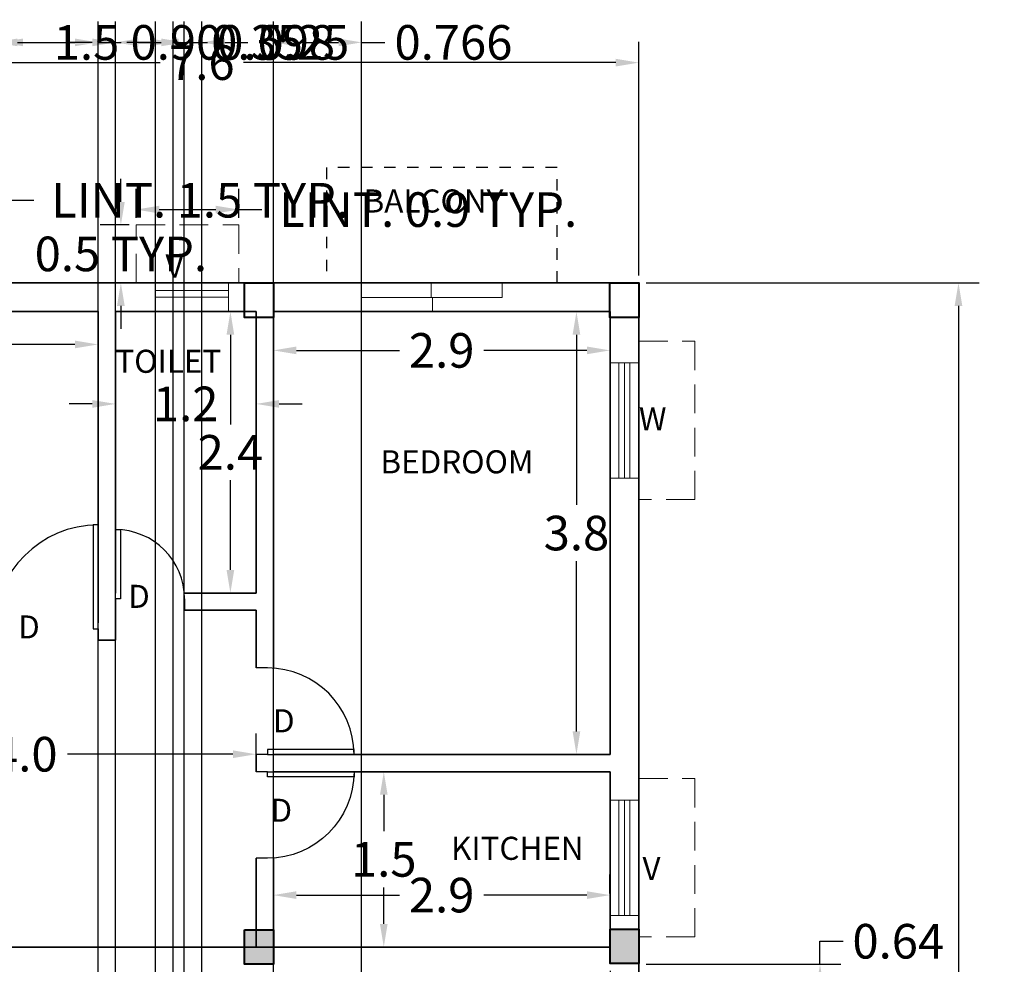
# Model space of a CAD drawing. Units: metres. Extents: x 106.5 to 121.4, y 89.1 to 111.8.
# Tile 5 of 5: x 112.4 to 121, y 103.6 to 111.8. Entities that reach past the tile are written whole.
import ezdxf

# ---------------------------------------------------------------- set-up
doc = ezdxf.new("R2010")
doc.units = ezdxf.units.M
doc.header["$MEASUREMENT"] = 0
doc.linetypes.add('ACAD_ISO07W100', pattern=[3, 0, -3])
doc.linetypes.add('HIDDEN', pattern=[0.375, 0.25, -0.125])
doc.layers.get('0').update_dxf_attribs({"color": 1})
for name, color, linetype, lineweight in [('A-ANNO-DIMS', 5, 'Continuous', 18), ('A-ANNO-TEXT', 4, 'Continuous', 18), ('A-AREA-IDEN', 4, 'Continuous', 18), ('A-COLS-PATT', 18, 'Continuous', 13), ('A-FLOR-BALC', 240, 'ACAD_ISO07W100', 25), ('A-WALL', 1, 'Continuous', 35), ('COLUMN', 244, 'Continuous', 40), ('DR', 2, 'Continuous', 25), ('LNTL', 240, 'HIDDEN', 18), ('VNTLTR', 8, 'Continuous', 18), ('WNDW', 3, 'Continuous', 18)]:
    doc.layers.add(name, color=color, linetype=linetype, lineweight=lineweight)
doc.styles.get("Standard").update_dxf_attribs({"font": 'arial.ttf'})
doc.dimstyles.get("Standard").update_dxf_attribs({"dimtxt": 0.3, "dimasz": 0.2, "dimexe": 0.18, "dimexo": 0.0625, "dimgap": 0.09, "dimtad": 0, "dimtih": 1, "dimtoh": 1, "dimdec": 1, "dimzin": 0, "dimdsep": 46, "dimtxsty": 'Standard', "dimcen": 0.09, "dimadec": 0, "dimazin": 0, "dimtfac": 1, "dimtdec": 1, "dimtofl": 0, "dimtmove": 0, "dimatfit": 3, "dimfxl": 1, "dimtolj": 1, "dimtzin": 0, "dimarcsym": 0})

# ---------------------------------------------------------------- blocks, each defined once
blk = doc.blocks.new('*U2')
for p, q in [((0, 0), (0, -100)), ((-900, 0), (-900, -100))]:
    blk.add_line(p, q)
blk.add_lwpolyline([(0, 0), (0, 900), (-43.75, 900), (-43.75, 0)], close=True)
blk.add_arc((0, 0), 900, 90, 180)
blk = doc.blocks.new('*U3')
for p, q in [((0, 0), (0, -100)), ((600, 0), (600, -100))]:
    blk.add_line(p, q)
blk.add_lwpolyline([(0, 0), (0, 600), (43.75, 600), (43.75, 0)], close=True)
blk.add_arc((0, 0), 600, 0, 90)
blk = doc.blocks.new('*U4')
for p, q in [((-750, 0), (-750, -100)), ((0, 0), (0, -100))]:
    blk.add_line(p, q)
blk.add_lwpolyline([(0, 0), (0, 750), (-43.75, 750), (-43.75, 0)], close=True)
blk.add_arc((0, 0), 750, 90, 180)
blk = doc.blocks.new('*D7')
at = {"layer": 'A-ANNO-DIMS', "color": 0, "lineweight": -2, "ltscale": 0.5, "transparency": 16777216}
for p, q in [((110.2029, 109.5663), (110.2029, 111.5934)), ((117.7829, 109.5663), (117.7829, 111.5934)), ((110.4029, 111.4134), (113.6312, 111.4134)), ((117.5829, 111.4134), (114.3547, 111.4134))]:
    blk.add_line(p, q, dxfattribs=at)
at = {"layer": 'A-ANNO-DIMS', "color": 0, "lineweight": -3, "ltscale": 0.5, "transparency": 16777216}
for points in [[(110.4029, 111.4467), (110.4029, 111.3801), (110.2029, 111.4134)], [(117.5829, 111.4467), (117.5829, 111.3801), (117.7829, 111.4134)]]:
    blk.add_solid(points, dxfattribs=at)
at = {"layer": 'Defpoints', "color": 0, "lineweight": -3, "ltscale": 0.5, "transparency": 16777216}
for p in [(117.7829, 111.4134), (110.2029, 109.5038), (117.7829, 109.5038)]:
    blk.add_point(p, dxfattribs=at)
at = {"layer": 'A-ANNO-DIMS', "color": 0, "ltscale": 0.5, "transparency": 16777216, "insert": (113.9929, 111.4134), "char_height": 0.3, "attachment_point": 5}
blk.add_mtext('\\A1;7.6', dxfattribs=at)
blk = doc.blocks.new('*D9')
at = {"layer": 'A-ANNO-DIMS', "color": 0, "lineweight": -2, "ltscale": 0.5, "transparency": 16777216}
for p, q in [((112.2429, 103.5313), (112.2429, 102.5093)), ((117.5329, 103.5371), (117.5329, 102.5093)), ((112.4429, 102.6893), (114.5248, 102.6893)), ((117.3329, 102.6893), (115.251, 102.6893))]:
    blk.add_line(p, q, dxfattribs=at)
at = {"layer": 'A-ANNO-DIMS', "color": 0, "lineweight": -3, "ltscale": 0.5, "transparency": 16777216}
for points in [[(112.4429, 102.7226), (112.4429, 102.6559), (112.2429, 102.6893)], [(117.3329, 102.7226), (117.3329, 102.6559), (117.5329, 102.6893)]]:
    blk.add_solid(points, dxfattribs=at)
at = {"layer": 'Defpoints', "color": 0, "lineweight": -3, "ltscale": 0.5, "transparency": 16777216}
for p in [(112.2429, 103.5938), (117.5329, 103.5996), (117.5329, 102.6893)]:
    blk.add_point(p, dxfattribs=at)
at = {"layer": 'A-ANNO-DIMS', "color": 0, "ltscale": 0.5, "transparency": 16777216, "insert": (114.8879, 102.6893), "char_height": 0.3, "attachment_point": 5}
blk.add_mtext('\\A1;5.3', dxfattribs=at)
blk = doc.blocks.new('*D12')
at = {"layer": 'A-ANNO-DIMS', "color": 0, "lineweight": -2, "ltscale": 0.5, "transparency": 16777216}
for p, q in [((114.6129, 104.209), (114.6129, 104.3739)), ((117.5322, 104.209), (117.5322, 104.3739)), ((114.8129, 104.1939), (115.7066, 104.1939)), ((117.3322, 104.1939), (116.4385, 104.1939))]:
    blk.add_line(p, q, dxfattribs=at)
at = {"layer": 'A-ANNO-DIMS', "color": 0, "lineweight": -3, "ltscale": 0.5, "transparency": 16777216}
for points in [[(114.8129, 104.2272), (114.8129, 104.1606), (114.6129, 104.1939)], [(117.3322, 104.2272), (117.3322, 104.1606), (117.5322, 104.1939)]]:
    blk.add_solid(points, dxfattribs=at)
at = {"layer": 'Defpoints', "color": 0, "lineweight": -3, "ltscale": 0.5, "transparency": 16777216}
for p in [(117.5322, 104.1939), (114.6129, 104.1465), (117.5322, 104.1465)]:
    blk.add_point(p, dxfattribs=at)
at = {"layer": 'A-ANNO-DIMS', "color": 0, "ltscale": 0.5, "transparency": 16777216, "insert": (116.0725, 104.1939), "char_height": 0.3, "attachment_point": 5}
blk.add_mtext('\\A1;2.9', dxfattribs=at)
blk = doc.blocks.new('*D13')
at = {"layer": 'A-ANNO-DIMS', "color": 0, "lineweight": -2, "ltscale": 0.5, "transparency": 16777216}
for p, q in [((115.6333, 105.2638), (115.7508, 105.2638)), ((115.5708, 105.0638), (115.5708, 104.747)), ((115.5708, 103.9438), (115.5708, 104.2606)), ((115.6333, 103.7438), (115.7508, 103.7438))]:
    blk.add_line(p, q, dxfattribs=at)
at = {"layer": 'A-ANNO-DIMS', "color": 0, "lineweight": -3, "ltscale": 0.5, "transparency": 16777216}
for points in [[(115.5375, 105.0638), (115.6041, 105.0638), (115.5708, 105.2638)], [(115.5375, 103.9438), (115.6041, 103.9438), (115.5708, 103.7438)]]:
    blk.add_solid(points, dxfattribs=at)
at = {"layer": 'Defpoints', "color": 0, "lineweight": -3, "ltscale": 0.5, "transparency": 16777216}
for p in [(115.5708, 105.2638), (115.5708, 103.7438), (115.5708, 103.7438)]:
    blk.add_point(p, dxfattribs=at)
at = {"layer": 'A-ANNO-DIMS', "color": 0, "ltscale": 0.5, "transparency": 16777216, "insert": (115.5708, 104.5038), "char_height": 0.3, "attachment_point": 5}
blk.add_mtext('\\A1;1.5', dxfattribs=at)
blk = doc.blocks.new('*D14')
at = {"layer": 'A-ANNO-DIMS', "color": 0, "lineweight": -2, "ltscale": 0.5, "transparency": 16777216}
for p, q in [((117.3039, 109.2538), (117.4214, 109.2538)), ((117.2414, 109.0538), (117.2414, 107.5771)), ((117.2414, 105.6138), (117.2414, 107.0905)), ((117.3039, 105.4138), (117.4214, 105.4138))]:
    blk.add_line(p, q, dxfattribs=at)
at = {"layer": 'A-ANNO-DIMS', "color": 0, "lineweight": -3, "ltscale": 0.5, "transparency": 16777216}
for points in [[(117.2081, 109.0538), (117.2747, 109.0538), (117.2414, 109.2538)], [(117.2081, 105.6138), (117.2747, 105.6138), (117.2414, 105.4138)]]:
    blk.add_solid(points, dxfattribs=at)
at = {"layer": 'Defpoints', "color": 0, "lineweight": -3, "ltscale": 0.5, "transparency": 16777216}
for p in [(117.2414, 109.2538), (117.2414, 105.4138), (117.2414, 105.4138)]:
    blk.add_point(p, dxfattribs=at)
at = {"layer": 'A-ANNO-DIMS', "color": 0, "ltscale": 0.5, "transparency": 16777216, "insert": (117.2414, 107.3338), "char_height": 0.3, "attachment_point": 5}
blk.add_mtext('\\A1;3.8', dxfattribs=at)
blk = doc.blocks.new('*D15')
at = {"layer": 'A-ANNO-DIMS', "color": 0, "lineweight": -2, "ltscale": 0.5, "transparency": 16777216}
for p, q in [((114.6129, 108.9803), (114.6129, 109.0978)), ((117.5329, 108.9803), (117.5329, 109.0978)), ((114.8129, 108.9178), (115.707, 108.9178)), ((117.3329, 108.9178), (116.4389, 108.9178))]:
    blk.add_line(p, q, dxfattribs=at)
at = {"layer": 'A-ANNO-DIMS', "color": 0, "lineweight": -3, "ltscale": 0.5, "transparency": 16777216}
for points in [[(114.8129, 108.9512), (114.8129, 108.8845), (114.6129, 108.9178)], [(117.3329, 108.9512), (117.3329, 108.8845), (117.5329, 108.9178)]]:
    blk.add_solid(points, dxfattribs=at)
at = {"layer": 'Defpoints', "color": 0, "lineweight": -3, "ltscale": 0.5, "transparency": 16777216}
for p in [(114.6129, 108.9178), (117.5329, 108.9178), (117.5329, 108.9178)]:
    blk.add_point(p, dxfattribs=at)
at = {"layer": 'A-ANNO-DIMS', "color": 0, "ltscale": 0.5, "transparency": 16777216, "insert": (116.0729, 108.9178), "char_height": 0.3, "attachment_point": 5}
blk.add_mtext('\\A1;2.9', dxfattribs=at)
blk = doc.blocks.new('*D16')
at = {"layer": 'A-ANNO-DIMS', "color": 0, "lineweight": -2, "ltscale": 0.5, "transparency": 16777216}
for p, q in [((113.0429, 108.4536), (112.8429, 108.4536)), ((113.2429, 108.5235), (113.2429, 108.2736)), ((114.4629, 108.5235), (114.4629, 108.2736)), ((114.6629, 108.4536), (114.8629, 108.4536))]:
    blk.add_line(p, q, dxfattribs=at)
at = {"layer": 'A-ANNO-DIMS', "color": 0, "lineweight": -3, "ltscale": 0.5, "transparency": 16777216}
for points in [[(113.0429, 108.4869), (113.0429, 108.4203), (113.2429, 108.4536)], [(114.6629, 108.4869), (114.6629, 108.4203), (114.4629, 108.4536)]]:
    blk.add_solid(points, dxfattribs=at)
at = {"layer": 'Defpoints', "color": 0, "lineweight": -3, "ltscale": 0.5, "transparency": 16777216}
for p in [(113.2429, 108.586), (114.4629, 108.586), (114.4629, 108.4536)]:
    blk.add_point(p, dxfattribs=at)
at = {"layer": 'A-ANNO-DIMS', "color": 0, "ltscale": 0.5, "transparency": 16777216, "insert": (113.8529, 108.4536), "char_height": 0.3, "attachment_point": 5}
blk.add_mtext('\\A1;1.2', dxfattribs=at)
blk = doc.blocks.new('*D17')
at = {"layer": 'A-ANNO-DIMS', "color": 0, "lineweight": -2, "ltscale": 0.5, "transparency": 16777216}
for p, q in [((114.3007, 109.2538), (114.0607, 109.2538)), ((114.2407, 109.0538), (114.2407, 108.2744)), ((114.2407, 107.0138), (114.2407, 107.7932)), ((114.3007, 106.8138), (114.0607, 106.8138))]:
    blk.add_line(p, q, dxfattribs=at)
at = {"layer": 'A-ANNO-DIMS', "color": 0, "lineweight": -3, "ltscale": 0.5, "transparency": 16777216}
for points in [[(114.2073, 109.0538), (114.274, 109.0538), (114.2407, 109.2538)], [(114.2073, 107.0138), (114.274, 107.0138), (114.2407, 106.8138)]]:
    blk.add_solid(points, dxfattribs=at)
at = {"layer": 'Defpoints', "color": 0, "lineweight": -3, "ltscale": 0.5, "transparency": 16777216}
for p in [(114.3632, 109.2538), (114.2407, 106.8138), (114.3632, 106.8138)]:
    blk.add_point(p, dxfattribs=at)
at = {"layer": 'A-ANNO-DIMS', "color": 0, "ltscale": 0.5, "transparency": 16777216, "insert": (114.2407, 108.0338), "char_height": 0.3, "attachment_point": 5}
blk.add_mtext('\\A1;2.4', dxfattribs=at)
blk = doc.blocks.new('*D18')
at = {"layer": 'A-ANNO-DIMS', "color": 0, "lineweight": -2, "ltscale": 0.5, "transparency": 16777216}
for p, q in [((110.4529, 109.0319), (110.4529, 109.1494)), ((113.0929, 109.0319), (113.0929, 109.1494)), ((110.6529, 108.9694), (111.4074, 108.9694)), ((112.8929, 108.9694), (112.1385, 108.9694))]:
    blk.add_line(p, q, dxfattribs=at)
at = {"layer": 'A-ANNO-DIMS', "color": 0, "lineweight": -3, "ltscale": 0.5, "transparency": 16777216}
for points in [[(110.6529, 109.0028), (110.6529, 108.9361), (110.4529, 108.9694)], [(112.8929, 109.0028), (112.8929, 108.9361), (113.0929, 108.9694)]]:
    blk.add_solid(points, dxfattribs=at)
at = {"layer": 'Defpoints', "color": 0, "lineweight": -3, "ltscale": 0.5, "transparency": 16777216}
for p in [(110.4529, 108.9694), (113.0929, 108.9694), (113.0929, 108.9694)]:
    blk.add_point(p, dxfattribs=at)
at = {"layer": 'A-ANNO-DIMS', "color": 0, "ltscale": 0.5, "transparency": 16777216, "insert": (111.7729, 108.9694), "char_height": 0.3, "attachment_point": 5}
blk.add_mtext('\\A1;2.6', dxfattribs=at)
blk = doc.blocks.new('*D20')
at = {"layer": 'A-ANNO-DIMS', "color": 0, "lineweight": -2, "ltscale": 0.5, "transparency": 16777216}
for p, q in [((110.4529, 105.4011), (110.4529, 105.5958)), ((114.4629, 105.4011), (114.4629, 105.5958)), ((110.6529, 105.4158), (112.0893, 105.4158)), ((114.2629, 105.4158), (112.8265, 105.4158))]:
    blk.add_line(p, q, dxfattribs=at)
at = {"layer": 'A-ANNO-DIMS', "color": 0, "lineweight": -3, "ltscale": 0.5, "transparency": 16777216}
for points in [[(110.6529, 105.4492), (110.6529, 105.3825), (110.4529, 105.4158)], [(114.2629, 105.4492), (114.2629, 105.3825), (114.4629, 105.4158)]]:
    blk.add_solid(points, dxfattribs=at)
at = {"layer": 'Defpoints', "color": 0, "lineweight": -3, "ltscale": 0.5, "transparency": 16777216}
for p in [(110.4529, 105.4158), (110.4529, 105.3386), (114.4629, 105.3386)]:
    blk.add_point(p, dxfattribs=at)
at = {"layer": 'A-ANNO-DIMS', "color": 0, "ltscale": 0.5, "transparency": 16777216, "insert": (112.4579, 105.4158), "char_height": 0.3, "attachment_point": 5}
blk.add_mtext('\\A1;4.0', dxfattribs=at)
blk = doc.blocks.new('*D24')
at = {"layer": 'A-ANNO-DIMS', "color": 0, "lineweight": -2, "ltscale": 0.5, "transparency": 16777216}
for p, q in [((117.8454, 109.5038), (120.7343, 109.5038)), ((120.5543, 109.3038), (120.5543, 100.662)), ((120.5543, 91.5338), (120.5543, 100.1756)), ((117.8446, 91.3338), (120.7343, 91.3338))]:
    blk.add_line(p, q, dxfattribs=at)
at = {"layer": 'A-ANNO-DIMS', "color": 0, "lineweight": -3, "ltscale": 0.5, "transparency": 16777216}
for points in [[(120.521, 109.3038), (120.5876, 109.3038), (120.5543, 109.5038)], [(120.521, 91.5338), (120.5876, 91.5338), (120.5543, 91.3338)]]:
    blk.add_solid(points, dxfattribs=at)
at = {"layer": 'Defpoints', "color": 0, "lineweight": -3, "ltscale": 0.5, "transparency": 16777216}
for p in [(117.7829, 109.5038), (117.7821, 91.3338), (120.5543, 91.3338)]:
    blk.add_point(p, dxfattribs=at)
at = {"layer": 'A-ANNO-DIMS', "color": 0, "ltscale": 0.5, "transparency": 16777216, "insert": (120.5543, 100.4188), "char_height": 0.3, "attachment_point": 5}
blk.add_mtext('\\A1;18.2', dxfattribs=at)
blk = doc.blocks.new('WIN-1000-SIDE')
for p, q in [((0.0782, 0.9998), (0.0782, -0.0002)), ((0.1249, 0.9998), (0.1249, -0.0002)), ((0.1718, -0.0002), (0.1718, 0.9998))]:
    blk.add_line(p, q)
blk.add_lwpolyline([(-0.0001, 0.9998), (0.2499, 0.9998), (0.2499, -0.0002), (-0.0001, -0.0002)], close=True)
blk = doc.blocks.new('BALCONY-SLIDING-LIGHT')
for points in [[(0.6038, 0.2498), (1.217, 0.2498), (1.217, 0.1224), (0.6014, 0.1224)], [(-0.0001, -0.0002), (0.613, -0.0002), (0.613, 0.1224), (-0.0001, 0.1224)]]:
    blk.add_lwpolyline(points, close=True)
blk = doc.blocks.new('VENT-0634')
for p, q in [((-0.0005, 0.1839), (0.6339, 0.1839)), ((-0.0005, 0.1248), (0.6339, 0.1248))]:
    blk.add_line(p, q)
blk.add_lwpolyline([(-0.0005, 0.2498), (0.6339, 0.2498), (0.6339, -0.0002), (-0.0005, -0.0002)], close=True)
blk = doc.blocks.new('LINTEL-PROJ-1373')
for p, q in [((-0.0001, 1.3733), (0.4855, 1.3733)), ((0.4855, 1.3733), (0.4855, 0.0001)), ((0.4855, 0.0001), (-0.0001, 0.0001))]:
    blk.add_line(p, q)
blk = doc.blocks.new('LINTEL-PROJ-0890')
for p, q in [((0.0002, -0.0002), (0.0002, 0.5015)), ((0.0002, 0.5015), (0.8897, 0.5015)), ((0.8897, 0.5015), (0.8897, -0.0002))]:
    blk.add_line(p, q)
blk = doc.blocks.new('BALCONY-2000X1000')
at = {"ltscale": 0.02}
blk.add_lwpolyline([(-0.0001, -0.0002), (1.9999, -0.0002), (1.9999, 0.9998), (-0.0001, 0.9998)], close=True, dxfattribs=at)
blk = doc.blocks.new('COL-250X300')
at = {"ltscale": 0.5}
blk.add_lwpolyline([(-0.0001, 0.2999), (0.2499, 0.2999), (0.2499, -0.0001), (-0.0001, -0.0001)], close=True, dxfattribs=at)
blk = doc.blocks.new('*D43')
at = {"layer": 'A-ANNO-DIMS', "color": 0, "lineweight": -2, "ltscale": 0.5, "transparency": 16777216}
for p, q in [((117.5254, 103.0171), (117.5254, 103.5072)), ((117.7754, 103.0171), (117.7754, 103.5072)), ((117.3254, 103.3272), (117.1254, 103.3272)), ((117.9754, 103.3272), (118.1754, 103.3272))]:
    blk.add_line(p, q, dxfattribs=at)
at = {"layer": 'A-ANNO-DIMS', "color": 0, "lineweight": -3, "ltscale": 0.5, "transparency": 16777216}
for points in [[(117.3254, 103.3605), (117.3254, 103.2939), (117.5254, 103.3272)], [(117.9754, 103.3605), (117.9754, 103.2939), (117.7754, 103.3272)]]:
    blk.add_solid(points, dxfattribs=at)
at = {"layer": 'Defpoints', "color": 0, "lineweight": -3, "ltscale": 0.5, "transparency": 16777216}
for p in [(117.7754, 103.3272), (117.5254, 102.9546), (117.7754, 102.9546)]:
    blk.add_point(p, dxfattribs=at)
at = {"layer": 'A-ANNO-DIMS', "color": 0, "ltscale": 0.5, "transparency": 16777216, "insert": (119.0537, 103.3272), "char_height": 0.3, "attachment_point": 5}
blk.add_mtext('\\A1;0.3 TYP.', dxfattribs=at)
blk = doc.blocks.new('*D52')
at = {"layer": 'A-ANNO-DIMS', "color": 0, "lineweight": -2, "ltscale": 0.5, "transparency": 16777216}
for p, q in [((110.8805, 110.0641), (110.8805, 110.3999)), ((112.3357, 110.0641), (112.3357, 110.3999)), ((111.0805, 110.2199), (112.1357, 110.2199)), ((112.3357, 110.2199), (112.5357, 110.2199))]:
    blk.add_line(p, q, dxfattribs=at)
at = {"layer": 'A-ANNO-DIMS', "color": 0, "lineweight": -3, "ltscale": 0.5, "transparency": 16777216}
for points in [[(111.0805, 110.2532), (111.0805, 110.1865), (110.8805, 110.2199)], [(112.1357, 110.2532), (112.1357, 110.1865), (112.3357, 110.2199)]]:
    blk.add_solid(points, dxfattribs=at)
at = {"layer": 'Defpoints', "color": 0, "lineweight": -3, "ltscale": 0.5, "transparency": 16777216}
for p in [(112.3357, 110.2199), (110.8805, 110.0016), (112.3357, 110.0016)]:
    blk.add_point(p, dxfattribs=at)
at = {"layer": 'A-ANNO-DIMS', "color": 0, "ltscale": 0.5, "transparency": 16777216, "insert": (113.978, 110.2199), "char_height": 0.3, "attachment_point": 5}
blk.add_mtext('\\A1;LINT. 1.5 TYP.', dxfattribs=at)
blk = doc.blocks.new('*D54')
at = {"layer": 'A-ANNO-DIMS', "color": 0, "lineweight": -2, "ltscale": 0.5, "transparency": 16777216}
for p, q in [((113.4242, 110.068), (113.4242, 110.3189)), ((114.3137, 110.068), (114.3137, 110.3189)), ((113.6242, 110.1389), (114.1137, 110.1389)), ((114.3137, 110.1389), (114.5137, 110.1389))]:
    blk.add_line(p, q, dxfattribs=at)
at = {"layer": 'A-ANNO-DIMS', "color": 0, "lineweight": -3, "ltscale": 0.5, "transparency": 16777216}
for points in [[(113.6242, 110.1722), (113.6242, 110.1056), (113.4242, 110.1389)], [(114.1137, 110.1722), (114.1137, 110.1056), (114.3137, 110.1389)]]:
    blk.add_solid(points, dxfattribs=at)
at = {"layer": 'Defpoints', "color": 0, "lineweight": -3, "ltscale": 0.5, "transparency": 16777216}
for p in [(114.3137, 110.1389), (113.4242, 110.0055), (114.3137, 110.0055)]:
    blk.add_point(p, dxfattribs=at)
at = {"layer": 'A-ANNO-DIMS', "color": 0, "ltscale": 0.5, "transparency": 16777216, "insert": (115.956, 110.1389), "char_height": 0.3, "attachment_point": 5}
blk.add_mtext('\\A1;LINT. 0.9 TYP.', dxfattribs=at)
blk = doc.blocks.new('*D55')
at = {"layer": 'A-ANNO-DIMS', "color": 0, "lineweight": -2, "ltscale": 0.5, "transparency": 16777216}
for p, q in [((113.2908, 110.2055), (113.2908, 110.4055)), ((113.3617, 110.0055), (113.1108, 110.0055)), ((113.3617, 109.5038), (113.1108, 109.5038)), ((113.2908, 109.3038), (113.2908, 109.1038))]:
    blk.add_line(p, q, dxfattribs=at)
at = {"layer": 'A-ANNO-DIMS', "color": 0, "lineweight": -3, "ltscale": 0.5, "transparency": 16777216}
for points in [[(113.2574, 110.2055), (113.3241, 110.2055), (113.2908, 110.0055)], [(113.2574, 109.3038), (113.3241, 109.3038), (113.2908, 109.5038)]]:
    blk.add_solid(points, dxfattribs=at)
at = {"layer": 'Defpoints', "color": 0, "lineweight": -3, "ltscale": 0.5, "transparency": 16777216}
for p in [(113.2908, 110.0055), (113.4242, 110.0055), (113.4242, 109.5038)]:
    blk.add_point(p, dxfattribs=at)
at = {"layer": 'A-ANNO-DIMS', "color": 0, "ltscale": 0.5, "transparency": 16777216, "insert": (113.2908, 109.7546), "char_height": 0.3, "attachment_point": 5}
blk.add_mtext('\\A1;0.5 TYP.', dxfattribs=at)
blk = doc.blocks.new('*D59')
at = {"layer": 'A-ANNO-DIMS', "color": 0, "lineweight": -2, "ltscale": 0.5, "transparency": 16777216}
for p, q in [((112.1943, 94.3463), (112.1943, 111.7688)), ((113.0929, 94.3463), (113.0929, 111.7688)), ((112.3943, 111.5888), (112.8929, 111.5888)), ((113.0929, 111.5888), (113.2929, 111.5888))]:
    blk.add_line(p, q, dxfattribs=at)
at = {"layer": 'A-ANNO-DIMS', "color": 0, "lineweight": -3, "ltscale": 0.5, "transparency": 16777216}
for points in [[(112.3943, 111.6221), (112.3943, 111.5555), (112.1943, 111.5888)], [(112.8929, 111.6221), (112.8929, 111.5555), (113.0929, 111.5888)]]:
    blk.add_solid(points, dxfattribs=at)
at = {"layer": 'Defpoints', "color": 0, "lineweight": -3, "ltscale": 0.5, "transparency": 16777216}
for p in [(113.0929, 111.5888), (112.1943, 94.2838), (113.0929, 94.2838)]:
    blk.add_point(p, dxfattribs=at)
at = {"layer": 'A-ANNO-DIMS', "color": 0, "ltscale": 0.5, "transparency": 16777216, "insert": (113.772, 111.5888), "char_height": 0.3, "attachment_point": 5}
blk.add_mtext('\\A1;0.90', dxfattribs=at)
blk = doc.blocks.new('*D60')
at = {"layer": 'A-ANNO-DIMS', "color": 0, "lineweight": -2, "ltscale": 0.5, "transparency": 16777216}
for p, q in [((113.2429, 94.0863), (113.2429, 111.7688)), ((113.8408, 94.0863), (113.8408, 111.7688)), ((113.4429, 111.5888), (113.6408, 111.5888)), ((113.8408, 111.5888), (114.0408, 111.5888))]:
    blk.add_line(p, q, dxfattribs=at)
at = {"layer": 'A-ANNO-DIMS', "color": 0, "lineweight": -3, "ltscale": 0.5, "transparency": 16777216}
for points in [[(113.4429, 111.6221), (113.4429, 111.5555), (113.2429, 111.5888)], [(113.6408, 111.6221), (113.6408, 111.5555), (113.8408, 111.5888)]]:
    blk.add_solid(points, dxfattribs=at)
at = {"layer": 'Defpoints', "color": 0, "lineweight": -3, "ltscale": 0.5, "transparency": 16777216}
for p in [(113.8408, 111.5888), (113.2429, 94.0238), (113.8408, 94.0238)]:
    blk.add_point(p, dxfattribs=at)
at = {"layer": 'A-ANNO-DIMS', "color": 0, "ltscale": 0.5, "transparency": 16777216, "insert": (114.6373, 111.5888), "char_height": 0.3, "attachment_point": 5}
blk.add_mtext('\\A1;0.598', dxfattribs=at)
blk = doc.blocks.new('*D64')
at = {"layer": 'A-ANNO-DIMS', "color": 0, "lineweight": -2, "ltscale": 0.5, "transparency": 16777216}
for p, q in [((113.2429, 91.6463), (113.2429, 111.7688)), ((113.5905, 91.6463), (113.5905, 111.7688)), ((113.0429, 111.5888), (112.8429, 111.5888)), ((113.7905, 111.5888), (113.9905, 111.5888))]:
    blk.add_line(p, q, dxfattribs=at)
at = {"layer": 'A-ANNO-DIMS', "color": 0, "lineweight": -3, "ltscale": 0.5, "transparency": 16777216}
for points in [[(113.0429, 111.6221), (113.0429, 111.5555), (113.2429, 111.5888)], [(113.7905, 111.6221), (113.7905, 111.5555), (113.5905, 111.5888)]]:
    blk.add_solid(points, dxfattribs=at)
at = {"layer": 'Defpoints', "color": 0, "lineweight": -3, "ltscale": 0.5, "transparency": 16777216}
for p in [(113.5905, 111.5888), (113.2429, 91.5838), (113.5905, 91.5838)]:
    blk.add_point(p, dxfattribs=at)
at = {"layer": 'A-ANNO-DIMS', "color": 0, "ltscale": 0.5, "transparency": 16777216, "insert": (114.4713, 111.5888), "char_height": 0.3, "attachment_point": 5}
blk.add_mtext('\\A1;0.35', dxfattribs=at)
blk = doc.blocks.new('*D65')
at = {"layer": 'A-ANNO-DIMS', "color": 0, "lineweight": -2, "ltscale": 0.5, "transparency": 16777216}
for p, q in [((114.6129, 91.6463), (114.6129, 111.7688)), ((115.3789, 91.6463), (115.3789, 111.7688)), ((114.8129, 111.5888), (115.1789, 111.5888)), ((115.3789, 111.5888), (115.5789, 111.5888))]:
    blk.add_line(p, q, dxfattribs=at)
at = {"layer": 'A-ANNO-DIMS', "color": 0, "lineweight": -3, "ltscale": 0.5, "transparency": 16777216}
for points in [[(114.8129, 111.6221), (114.8129, 111.5555), (114.6129, 111.5888)], [(115.1789, 111.6221), (115.1789, 111.5555), (115.3789, 111.5888)]]:
    blk.add_solid(points, dxfattribs=at)
at = {"layer": 'Defpoints', "color": 0, "lineweight": -3, "ltscale": 0.5, "transparency": 16777216}
for p in [(115.3789, 111.5888), (114.6129, 91.5838), (115.3789, 91.5838)]:
    blk.add_point(p, dxfattribs=at)
at = {"layer": 'A-ANNO-DIMS', "color": 0, "ltscale": 0.5, "transparency": 16777216, "insert": (116.1749, 111.5888), "char_height": 0.3, "attachment_point": 5}
blk.add_mtext('\\A1;0.766', dxfattribs=at)
blk = doc.blocks.new('*D72')
at = {"layer": 'A-ANNO-DIMS', "color": 0, "lineweight": -2, "ltscale": 0.5, "transparency": 16777216}
for p, q in [((112.2429, 98.9563), (112.2429, 111.7688)), ((113.7429, 98.9563), (113.7429, 111.7688)), ((112.4429, 111.5888), (112.6428, 111.5888)), ((113.5429, 111.5888), (113.343, 111.5888))]:
    blk.add_line(p, q, dxfattribs=at)
at = {"layer": 'A-ANNO-DIMS', "color": 0, "lineweight": -3, "ltscale": 0.5, "transparency": 16777216}
for points in [[(112.4429, 111.6221), (112.4429, 111.5555), (112.2429, 111.5888)], [(113.5429, 111.6221), (113.5429, 111.5555), (113.7429, 111.5888)]]:
    blk.add_solid(points, dxfattribs=at)
at = {"layer": 'Defpoints', "color": 0, "lineweight": -3, "ltscale": 0.5, "transparency": 16777216}
for p in [(113.7429, 111.5888), (112.2429, 98.8938), (113.7429, 98.8938)]:
    blk.add_point(p, dxfattribs=at)
at = {"layer": 'A-ANNO-DIMS', "color": 0, "ltscale": 0.5, "transparency": 16777216, "insert": (112.9929, 111.5888), "char_height": 0.3, "attachment_point": 5}
blk.add_mtext('\\A1;1.5', dxfattribs=at)
blk = doc.blocks.new('*D75')
at = {"layer": 'A-ANNO-DIMS', "color": 0, "lineweight": -2, "ltscale": 0.5, "transparency": 16777216}
for p, q in [((119.3535, 103.5938), (119.3535, 103.7938)), ((119.3535, 103.7938), (119.5535, 103.7938)), ((117.8454, 103.5938), (119.5335, 103.5938)), ((119.3535, 103.1546), (119.3535, 103.3938)), ((117.8379, 102.9546), (119.5335, 102.9546))]:
    blk.add_line(p, q, dxfattribs=at)
at = {"layer": 'A-ANNO-DIMS', "color": 0, "lineweight": -3, "ltscale": 0.5, "transparency": 16777216}
for points in [[(119.3201, 103.3938), (119.3868, 103.3938), (119.3535, 103.5938)], [(119.3201, 103.1546), (119.3868, 103.1546), (119.3535, 102.9546)]]:
    blk.add_solid(points, dxfattribs=at)
at = {"layer": 'Defpoints', "color": 0, "lineweight": -3, "ltscale": 0.5, "transparency": 16777216}
for p in [(117.7829, 103.5938), (119.3535, 103.5938), (117.7754, 102.9546)]:
    blk.add_point(p, dxfattribs=at)
at = {"layer": 'A-ANNO-DIMS', "color": 0, "ltscale": 0.5, "transparency": 16777216, "insert": (120.0325, 103.7938), "char_height": 0.3, "attachment_point": 5}
blk.add_mtext('\\A1;0.64', dxfattribs=at)
blk = doc.blocks.new('*D76')
at = {"layer": 'A-ANNO-DIMS', "color": 0, "lineweight": -2, "ltscale": 0.5, "transparency": 16777216}
for p, q in [((113.7429, 101.5463), (113.7429, 111.7688)), ((113.9929, 101.5463), (113.9929, 111.7688)), ((113.5429, 111.5888), (113.3429, 111.5888)), ((114.1929, 111.5888), (114.3929, 111.5888))]:
    blk.add_line(p, q, dxfattribs=at)
at = {"layer": 'A-ANNO-DIMS', "color": 0, "lineweight": -3, "ltscale": 0.5, "transparency": 16777216}
for points in [[(113.5429, 111.6221), (113.5429, 111.5555), (113.7429, 111.5888)], [(114.1929, 111.6221), (114.1929, 111.5555), (113.9929, 111.5888)]]:
    blk.add_solid(points, dxfattribs=at)
at = {"layer": 'Defpoints', "color": 0, "lineweight": -3, "ltscale": 0.5, "transparency": 16777216}
for p in [(113.9929, 111.5888), (113.7429, 101.4838), (113.9929, 101.4838)]:
    blk.add_point(p, dxfattribs=at)
at = {"layer": 'A-ANNO-DIMS', "color": 0, "ltscale": 0.5, "transparency": 16777216, "insert": (114.8737, 111.5888), "char_height": 0.3, "attachment_point": 5}
blk.add_mtext('\\A1;0.25', dxfattribs=at)

msp = doc.modelspace()

# ---------------------------------------------------------------- hatches: boundary and pattern name
at = {"layer": 'A-COLS-PATT', "ltscale": 0.5}
h = msp.add_hatch(dxfattribs=at)
h.set_pattern_fill('CORK', color=256, scale=10)
h.set_pattern_definition([(0, (0, 0), (0, 1.25), []), (135, (0.625, -0.625), (-2.5, -2.5), [1.76777, -1.76777]), (135, (0.9375, -0.625), (-2.5, -2.5), [1.76777, -1.76777]), (135, (1.25, -0.625), (-2.5, -2.5), [1.76777, -1.76777])])
h.paths.add_polyline_path([(110.2029, 109.5038), (110.2029, 109.2038), (110.4529, 109.2038), (110.4529, 109.5038)])
h.paths.add_polyline_path([(114.6132, 109.5038), (114.3632, 109.5038), (114.3632, 109.2538), (114.4629, 109.2538), (114.4629, 109.2038), (114.6129, 109.2038), (114.6129, 109.2538)])
h.paths.add_polyline_path([(117.5321, 109.2538), (117.5329, 109.2538), (117.5329, 109.2038), (117.7821, 109.2038), (117.7821, 109.5038), (117.5321, 109.5038)])
h = msp.add_hatch(color=256, dxfattribs=at)
h.dxf.hatch_style = 1
h.paths.add_polyline_path([(110.4529, 103.8929), (110.2029, 103.8929), (110.2029, 103.5938), (110.4529, 103.5938)])
h.paths.add_polyline_path([(114.4629, 103.8938), (114.3632, 103.8938), (114.3632, 103.7438), (114.4629, 103.7438)])
h.paths.add_polyline_path([(114.6129, 103.8938), (114.4629, 103.8938), (114.4629, 103.7438), (114.6129, 103.7438)])
h.paths.add_polyline_path([(114.6132, 103.7438), (114.4629, 103.7438), (114.3632, 103.7438), (114.3632, 103.5938), (114.6132, 103.5938)])
h.paths.add_polyline_path([(117.7829, 103.8996), (117.5329, 103.8996), (117.5329, 103.5996), (117.7829, 103.5996)])
h.paths.add_polyline_path([(117.7829, 98.888), (117.5329, 98.888), (117.5329, 98.588), (117.7829, 98.588)])
h.paths.add_polyline_path([(110.4529, 98.8938), (110.2029, 98.8938), (110.2029, 98.5947), (110.4529, 98.5947)])
h.paths.add_polyline_path([(114.6132, 98.8938), (114.3132, 98.8938), (114.3132, 98.7438), (114.4632, 98.7438), (114.6132, 98.7438)])
h.paths.add_polyline_path([(110.4529, 91.6338), (110.2029, 91.6338), (110.2029, 91.3338), (110.4529, 91.3338)])
h.paths.add_polyline_path([(114.6132, 91.5838), (114.6129, 91.5838), (114.6129, 91.6338), (114.4629, 91.6338), (114.4629, 91.5838), (114.3632, 91.5838), (114.3632, 91.3338), (114.6132, 91.3338)])
h.paths.add_polyline_path([(117.7821, 91.6338), (117.5329, 91.6338), (117.5329, 91.5838), (117.5321, 91.3338), (117.7821, 91.3338)])

# ---------------------------------------------------------------- linework, layer by layer
at = {"layer": 'A-WALL'}
for p, q in [((117.7829, 109.5038), (110.2029, 109.5038)), ((117.7829, 101.3638), (117.7829, 109.5038)), ((113.0929, 109.2538), (110.4529, 109.2538)), ((113.0929, 109.2538), (113.0929, 106.5538)), ((113.2429, 109.2538), (113.2429, 106.8138)), ((114.4629, 109.2538), (113.2429, 109.2538)), ((114.4629, 109.2538), (114.4629, 106.8138)), ((117.5329, 109.2538), (114.6129, 109.2538)), ((114.6129, 109.2538), (114.6129, 106.1621)), ((117.5329, 105.4138), (117.5329, 109.2538)), ((114.4629, 106.8138), (113.8408, 106.8138)), ((113.2429, 106.6638), (113.2429, 106.4038)), ((114.4629, 106.6638), (113.8429, 106.6638)), ((114.4629, 106.6638), (114.4629, 106.1638)), ((114.4629, 105.4138), (114.4629, 105.2634)), ((117.5329, 105.4138), (114.6129, 105.4138)), ((117.5329, 105.2638), (114.6129, 105.2638)), ((114.6129, 105.2638), (114.6129, 105.2634)), ((117.5329, 103.7438), (117.5329, 105.2638)), ((114.4629, 104.5134), (114.4629, 103.7438)), ((114.6129, 104.5151), (114.6129, 103.7438)), ((114.6129, 103.7438), (111.4517, 103.7438)), ((117.5329, 103.7438), (114.6129, 103.7438))]:
    msp.add_line(p, q, dxfattribs=at)
at = {"layer": 'A-WALL', "ltscale": 0.5}
msp.add_line((113.0929, 106.4038), (113.2429, 106.4038), dxfattribs=at)
msp.add_line((113.0929, 106.4038), (113.2429, 106.4038), dxfattribs=at)
at = {"layer": 'COLUMN', "ltscale": 0.5}
for points in [[(114.3632, 109.5038), (114.6132, 109.5038), (114.6132, 109.2038), (114.3632, 109.2038)], [(117.5321, 109.5038), (117.7821, 109.5038), (117.7821, 109.2038), (117.5321, 109.2038)], [(117.5329, 103.8996), (117.7829, 103.8996), (117.7829, 103.5996), (117.5329, 103.5996)]]:
    msp.add_lwpolyline(points, close=True, dxfattribs=at)
at = {"layer": 'VNTLTR'}
for p, q in [((117.6105, 105.0185), (117.6105, 104.0185)), ((117.6572, 105.0185), (117.6572, 104.0185)), ((117.704, 104.0185), (117.704, 105.0185))]:
    msp.add_line(p, q, dxfattribs=at)
msp.add_lwpolyline([(117.5322, 105.0185), (117.7822, 105.0185), (117.7822, 104.0185), (117.5322, 104.0185)], close=True, dxfattribs=at)

# ---------------------------------------------------------------- block references
at = {"layer": 'A-FLOR-BALC'}
msp.add_blockref('BALCONY-2000X1000', (115.073, 109.504), dxfattribs=at)
at = {"layer": 'COLUMN'}
msp.add_blockref('COL-250X300', (114.3633, 103.5939), dxfattribs=at)
at = {"layer": 'DR', "xscale": 0.001, "yscale": 0.001, "zscale": 0.001}
for name, p in [('*U2', (113.0929, 106.5038)), ('*U3', (113.2429, 106.7638))]:
    msp.add_blockref(name, p, dxfattribs=at)
at = {"layer": 'DR', "yscale": 0.001, "zscale": 0.001, "rotation": 270}
for p, xscale in [((114.5629, 105.4138), 0.001), ((114.5629, 105.2634), -0.001)]:
    msp.add_blockref('*U4', p, dxfattribs=dict(at, xscale=xscale))
at = {"layer": 'LNTL'}
for name, p in [('LINTEL-PROJ-0890', (113.424, 109.504)), ('LINTEL-PROJ-1373', (117.783, 107.624)), ('LINTEL-PROJ-1373', (117.783, 103.8316))]:
    msp.add_blockref(name, p, dxfattribs=at)
at = {"layer": 'VNTLTR'}
msp.add_blockref('VENT-0634', (113.591, 109.254), dxfattribs=at)
at = {"layer": 'WNDW'}
for name, p in [('BALCONY-SLIDING-LIGHT', (115.379, 109.254)), ('WIN-1000-SIDE', (117.5322, 107.811))]:
    msp.add_blockref(name, p, dxfattribs=at)

# ---------------------------------------------------------------- texts
at = {"layer": 'A-ANNO-TEXT', "ltscale": 0.5, "char_height": 0.2, "attachment_point": 1}
for s, width, insert in [('V', 0.327871, (113.6775, 109.7498)), ('W', 0.390771, (117.7829, 108.4248)), ('D', 0.320447, (113.3537, 106.8847)), ('D', 0.320447, (112.3996, 106.6193)), ('D', 0.320447, (114.6098, 105.8056)), ('D', 0.320447, (114.5878, 105.0294)), ('V', 0.327871, (117.8138, 104.5252))]:
    msp.add_mtext_dynamic_manual_height_columns(s, width=width, gutter_width=1, heights=[0], dxfattribs=dict(at, insert=insert))
at = {"layer": 'A-AREA-IDEN', "ltscale": 0.5, "char_height": 0.2, "attachment_point": 1}
for s, width, insert in [('BALCONY', 0.825106, (115.3955, 110.3134)), ('TOILET', 0.904944, (113.2429, 108.9233)), ('BEDROOM', 0.914899, (115.5413, 108.0516)), ('KITCHEN', 0.914899, (116.1537, 104.6998))]:
    msp.add_mtext_dynamic_manual_height_columns(s, width=width, gutter_width=1, heights=[0], dxfattribs=dict(at, insert=insert))

# ---------------------------------------------------------------- dimensions: what is measured, and where the dimension line sits
at = {"layer": 'A-ANNO-DIMS', "ltscale": 0.5}
for base, p1, p2, override, picture, middle in [((113.0929, 111.5888), (112.1943, 94.2838), (113.0929, 94.2838), {"dimdec": 2, "dimlfac": 1, "dimrnd": 0, "dimzin": 0, "dimdsep": 46, "dimlunit": 2}, '*D59', (113.772, 111.5888)), ((113.7429, 111.5888), (112.2429, 98.8938), (113.7429, 98.8938), {"dimdec": 1, "dimlfac": 1, "dimrnd": 0, "dimzin": 0, "dimdsep": 46, "dimlunit": 2}, '*D72', (112.9929, 111.5888)), ((113.5905, 111.5888), (113.2429, 91.5838), (113.5905, 91.5838), {"dimdec": 2, "dimlfac": 1, "dimrnd": 0, "dimzin": 0, "dimdsep": 46, "dimlunit": 2}, '*D64', (114.4713, 111.5888)), ((113.8408, 111.5888), (113.2429, 94.0238), (113.8408, 94.0238), {"dimdec": 3, "dimlfac": 1, "dimrnd": 0, "dimzin": 0, "dimdsep": 46, "dimlunit": 2}, '*D60', (114.6373, 111.5888)), ((113.9929, 111.5888), (113.7429, 101.4838), (113.9929, 101.4838), {"dimdec": 2, "dimlfac": 1, "dimrnd": 0, "dimzin": 0, "dimdsep": 46, "dimlunit": 2}, '*D76', (114.8737, 111.5888)), ((115.3789, 111.5888), (114.6129, 91.5838), (115.3789, 91.5838), {"dimdec": 3, "dimlfac": 1, "dimrnd": 0, "dimzin": 0, "dimdsep": 46, "dimlunit": 2}, '*D65', (116.1749, 111.5888)), ((117.7829, 111.4134), (110.2029, 109.5038), (117.7829, 109.5038), {"dimclrd": 0, "dimclre": 0, "dimclrt": 0}, '*D7', (113.9929, 111.4134)), ((113.0929, 108.9694), (110.4529, 108.9694), (113.0929, 108.9694), {"dimclrd": 0, "dimclre": 0, "dimclrt": 0}, '*D18', (111.7729, 108.9694)), ((117.5329, 108.9178), (114.6129, 108.9178), (117.5329, 108.9178), {"dimclrd": 0, "dimclre": 0, "dimclrt": 0}, '*D15', (116.0729, 108.9178)), ((114.4629, 108.4536), (113.2429, 108.586), (114.4629, 108.586), {"dimclrd": 0, "dimclre": 0, "dimclrt": 0}, '*D16', (113.8529, 108.4536)), ((110.4529, 105.4158), (114.4629, 105.3386), (110.4529, 105.3386), {"dimclrd": 0, "dimclre": 0, "dimclrt": 0}, '*D20', (112.4579, 105.4158)), ((117.5322, 104.1939), (114.6129, 104.1465), (117.5322, 104.1465), {"dimclrd": 0, "dimclre": 0, "dimclrt": 0}, '*D12', (116.0725, 104.1939)), ((117.5329, 102.6893), (112.2429, 103.5938), (117.5329, 103.5996), {"dimclrd": 0, "dimclre": 0, "dimclrt": 0}, '*D9', (114.8879, 102.6893))]:
    dim = msp.add_linear_dim(base=base, p1=p1, p2=p2, dimstyle='Standard', override=override, dxfattribs=at)
    dim.commit()
    dim.dimension.update_dxf_attribs({"geometry": picture, "text_midpoint": middle})
for base, p1, p2, text, picture, middle in [((112.3357, 110.2199), (110.8805, 110.0016), (112.3357, 110.0016), 'LINT. <> TYP.', '*D52', (113.978, 110.2199)), ((114.3137, 110.1389), (113.4242, 110.0055), (114.3137, 110.0055), 'LINT. <> TYP.', '*D54', (115.956, 110.1389)), ((117.7753725261, 103.327206493), (117.5253725261, 102.9546403061), (117.7753725261, 102.9546403061), '<> TYP.', '*D43', (119.0537422396, 103.327206493))]:
    dim = msp.add_linear_dim(base=base, p1=p1, p2=p2, text=text, dimstyle='Standard', override={"dimdec": 1, "dimlfac": 1, "dimrnd": 0, "dimzin": 0, "dimdsep": 46, "dimlunit": 2}, dxfattribs=at)
    dim.commit()
    dim.dimension.update_dxf_attribs({"geometry": picture, "text_midpoint": middle})
dim = msp.add_linear_dim(base=(113.2908, 110.0055), p1=(113.4242, 109.5038), p2=(113.4242, 110.0055), angle=90, text='<> TYP.', dimstyle='Standard', override={"dimdec": 1, "dimlfac": 1, "dimrnd": 0, "dimzin": 0, "dimdsep": 46, "dimlunit": 2}, dxfattribs=at)
dim.commit()
dim.dimension.update_dxf_attribs({"geometry": '*D55', "text_midpoint": (113.2908, 109.7546)})
for base, p1, p2, override, picture, middle in [((120.5543, 91.3338), (117.7829, 109.5038), (117.7821, 91.3338), {"dimclrd": 0, "dimclre": 0, "dimclrt": 0}, '*D24', (120.5543, 100.4188)), ((114.2407, 106.8138), (114.3632, 109.2538), (114.3632, 106.8138), {"dimclrd": 0, "dimclre": 0, "dimclrt": 0}, '*D17', (114.2407, 108.0338)), ((117.2414, 105.4138), (117.2414, 109.2538), (117.2414, 105.4138), {"dimclrd": 0, "dimclre": 0, "dimclrt": 0}, '*D14', (117.2414, 107.3338)), ((115.5708, 103.7438), (115.5708, 105.2638), (115.5708, 103.7438), {"dimclrd": 0, "dimclre": 0, "dimclrt": 0}, '*D13', (115.5708, 104.5038)), ((119.3535, 103.5938), (117.7754, 102.9546), (117.7829, 103.5938), {"dimdec": 2, "dimlfac": 1, "dimrnd": 0, "dimzin": 0, "dimdsep": 46, "dimlunit": 2}, '*D75', (120.0325, 103.7938))]:
    dim = msp.add_linear_dim(base=base, p1=p1, p2=p2, angle=90, dimstyle='Standard', override=override, dxfattribs=at)
    dim.commit()
    dim.dimension.update_dxf_attribs({"geometry": picture, "text_midpoint": middle})

doc.saveas('drawing.dxf')
